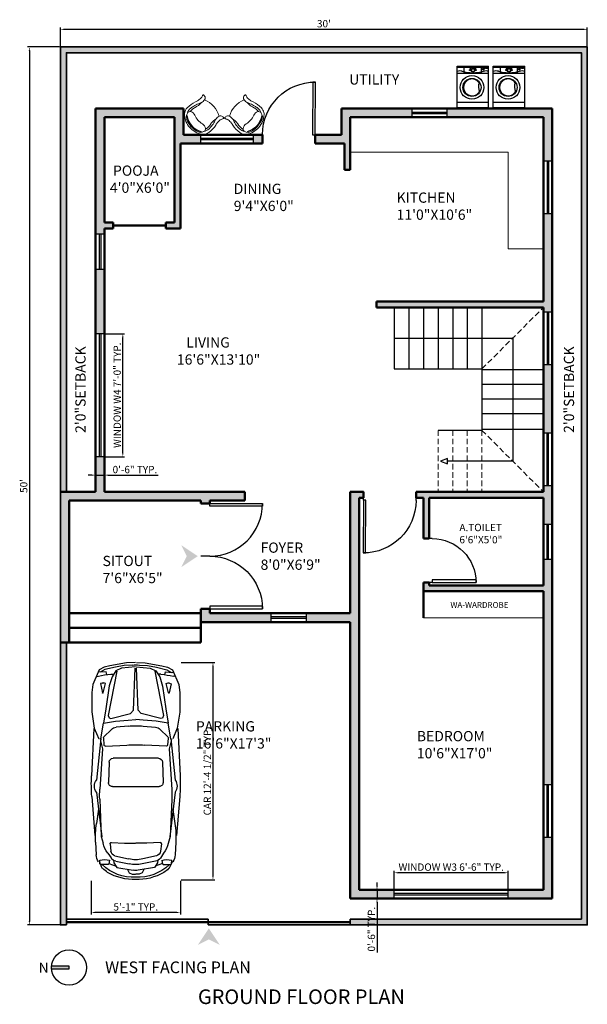
# Model space of a CAD drawing. Units: inches. Extents: x 2638 to 4577, y 1946 to 2619.
# Tile 7 of 8: x 3767 to 4155, y 1946 to 2619. Entities that reach past the tile are written whole.
import ezdxf

# ---------------------------------------------------------------- set-up
doc = ezdxf.new("R2010")
doc.units = ezdxf.units.IN
doc.linetypes.add('DASHED', pattern=[19.05, 12.7, -6.35])
for name, color, linetype, lineweight in [('A-ANNO-DIMS', 2, 'Continuous', 18), ('A-ANNO-SYMB', 1, 'Continuous', 25), ('A-ANNO-TEXT', 7, 'Continuous', 25), ('A-AREA-IDEN', 7, 'Continuous', 25), ('A-DOOR', 4, 'Continuous', 25), ('A-FLOR-FIXT', 8, 'Continuous', 18), ('A-FLOR-OVHD', 8, 'DASHED', 18), ('A-FLOR-STRS', 3, 'Continuous', 25), ('A-FURN', 8, 'Continuous', 18), ('A-GLAZ', 4, 'Continuous', 25), ('A-WALL', 7, 'Continuous', 50), ('A-WALL-PATT', 8, 'Continuous', 13), ('C-PROP', 1, 'Continuous', 35), ('C-PROP-PATT', 252, 'Continuous', 13)]:
    doc.layers.add(name, color=color, linetype=linetype, lineweight=lineweight)
for name, color, linetype in [('IFF-FURN-DETAIL', 250, 'Continuous'), ('L9012X$0', 2, 'Continuous'), ('Сантехника', 7, 'Continuous')]:
    doc.layers.add(name, color=color, linetype=linetype)
doc.styles.get("Standard").update_dxf_attribs({"font": 'arial.ttf'})
doc.dimstyles.new('ISO-25', dxfattribs={"dimtxt": 5, "dimasz": 2.5, "dimexe": 1.25, "dimexo": 0.625, "dimtad": 1, "dimdec": 1, "dimlunit": 3, "dimtxsty": 'Standard', "dimcen": 2.5, "dimclrt": 1, "dimadec": 0, "dimazin": 0, "dimtfac": 1, "dimtdec": 1, "dimtmove": 0, "dimatfit": 3, "dimfxl": 1, "dimarcsym": 0})

# ---------------------------------------------------------------- blocks, each defined once
blk = doc.blocks.new('*D39')
at = {"layer": 'A-ANNO-DIMS', "color": 0, "lineweight": -2, "transparency": 16777216}
for p, q in [((3795, 2600.78), (3795, 2613.44)), ((3797.5, 2612.19), (4152.5, 2612.19)), ((4155, 2600.78), (4155, 2613.44))]:
    blk.add_line(p, q, dxfattribs=at)
at = {"layer": 'A-ANNO-DIMS', "color": 0, "transparency": 16777216}
for points in [[(3797.5, 2612.61), (3797.5, 2611.77), (3795, 2612.19)], [(4152.5, 2612.61), (4152.5, 2611.77), (4155, 2612.19)]]:
    blk.add_solid(points, dxfattribs=at)
at = {"layer": 'Defpoints', "color": 0, "transparency": 16777216}
for p in [(4155, 2612.19), (3795, 2600.16), (4155, 2600.16)]:
    blk.add_point(p, dxfattribs=at)
at = {"layer": 'A-ANNO-DIMS', "color": 0, "transparency": 16777216, "insert": (3975, 2615.37), "char_height": 5, "attachment_point": 5}
blk.add_mtext("30'", dxfattribs=at)
blk = doc.blocks.new('*D40')
at = {"layer": 'A-ANNO-DIMS', "color": 0, "lineweight": -2, "transparency": 16777216}
for p, q in [((3794.38, 2600.16), (3772.46, 2600.16)), ((3773.71, 2597.66), (3773.71, 2002.66)), ((3794.38, 2000.16), (3772.46, 2000.16))]:
    blk.add_line(p, q, dxfattribs=at)
at = {"layer": 'A-ANNO-DIMS', "color": 0, "transparency": 16777216}
for points in [[(3773.29, 2597.66), (3774.12, 2597.66), (3773.71, 2600.16)], [(3773.29, 2002.66), (3774.12, 2002.66), (3773.71, 2000.16)]]:
    blk.add_solid(points, dxfattribs=at)
at = {"layer": 'Defpoints', "color": 0, "transparency": 16777216}
for p in [(3795, 2600.16), (3773.71, 2000.16), (3795, 2000.16)]:
    blk.add_point(p, dxfattribs=at)
at = {"layer": 'A-ANNO-DIMS', "color": 0, "transparency": 16777216, "insert": (3770.53, 2300.16), "char_height": 5, "attachment_point": 5, "rotation": 90}
blk.add_mtext("50'", dxfattribs=at)
blk = doc.blocks.new('*U5')
for p, q in [((0, 0), (0, -6)), ((30, 0), (30, -6))]:
    blk.add_line(p, q)
blk.add_lwpolyline([(0, 0), (0, 30), (1.75, 30), (1.75, 0)], close=True)
blk.add_arc((0, 0), 30, 0, 90)
blk = doc.blocks.new('*U4')
for p, q in [((0, 0), (0, -6)), ((36, 0), (36, -6))]:
    blk.add_line(p, q)
blk.add_lwpolyline([(0, 0), (0, 36), (1.75, 36), (1.75, 0)], close=True)
blk.add_arc((0, 0), 36, 0, 90)
blk = doc.blocks.new('wash')
at = {"layer": 'Сантехника'}
for p, q in [((4817.13, 2840.92), (4788.24, 2840.92)), ((4788.24, 2819.46), (4788.24, 2840.92)), ((4788.93, 2819.46), (4788.93, 2840.92)), ((4793.08, 2819.46), (4793.08, 2840.92)), ((4812.98, 2819.46), (4812.98, 2840.92)), ((4816.44, 2819.46), (4816.44, 2840.92)), ((4817.13, 2819.46), (4817.13, 2840.92)), ((4793.08, 2836.07), (4788.93, 2836.07)), ((4817.13, 2819.46), (4788.24, 2819.46)), ((4793.08, 2824.31), (4788.93, 2824.31)), ((4817.13, 2816.27), (4788.24, 2816.27)), ((4788.24, 2794.82), (4788.24, 2816.27)), ((4788.93, 2794.82), (4788.93, 2816.27)), ((4793.08, 2794.82), (4793.08, 2816.27)), ((4812.98, 2794.82), (4812.98, 2816.27)), ((4816.44, 2794.82), (4816.44, 2816.27)), ((4817.13, 2794.82), (4817.13, 2816.27)), ((4793.08, 2811.43), (4788.93, 2811.43)), ((4793.08, 2799.66), (4788.93, 2799.66)), ((4817.13, 2794.82), (4788.24, 2794.82))]:
    blk.add_line(p, q, dxfattribs=at)
for points in [[(4789.4, 2839.27), (4789.4, 2840.17), (4789.9, 2840.17), (4789.9, 2839.27)], [(4789.4, 2837.95), (4789.4, 2838.85), (4789.9, 2838.85), (4789.9, 2837.95)], [(4789.4, 2836.64), (4789.4, 2837.53), (4789.9, 2837.53), (4789.9, 2836.64)], [(4790.27, 2836.64), (4790.27, 2837.53), (4790.77, 2837.53), (4790.77, 2836.64)], [(4789.4, 2814.62), (4789.4, 2815.52), (4789.9, 2815.52), (4789.9, 2814.62)], [(4789.4, 2813.31), (4789.4, 2814.2), (4789.9, 2814.2), (4789.9, 2813.31)], [(4789.4, 2811.99), (4789.4, 2812.89), (4789.9, 2812.89), (4789.9, 2811.99)], [(4790.27, 2811.99), (4790.27, 2812.89), (4790.77, 2812.89), (4790.77, 2811.99)]]:
    blk.add_lwpolyline(points, close=True, dxfattribs=at)
for centre, radius in [((4802.77, 2829.54), 8.1), ((4802.77, 2829.54), 6.17), ((4789.46, 2831.45), 0.271), ((4789.46, 2828.92), 0.271), ((4790.98, 2830.19), 1.34), ((4790.19, 2831.93), 0.271), ((4790.98, 2830.19), 1.07), ((4790.19, 2828.4), 0.271), ((4790.98, 2832.18), 0.271), ((4790.98, 2828.15), 0.271), ((4802.77, 2804.9), 8.1), ((4789.46, 2806.8), 0.271), ((4790.98, 2805.55), 1.34), ((4790.19, 2807.28), 0.271), ((4790.98, 2805.55), 1.07), ((4790.98, 2807.53), 0.271), ((4802.77, 2804.9), 6.17), ((4789.46, 2804.27), 0.271), ((4790.19, 2803.75), 0.271), ((4790.98, 2803.5), 0.271)]:
    blk.add_circle(centre, radius, dxfattribs=at)
for centre, radius, start, end in [((4796.44, 2838.85), 4.89, 154.89498, 196.60684), ((4762.87, 2829.66), 29.92, 1.02061, 15.09365), ((4802.77, 2829.54), 5.77, 121.80671, 62.15064), ((4802.39, 2840.74), 6.83, 243.19, 300.76734), ((4762.87, 2830.72), 29.92, 344.90635, 358.97939), ((4796.44, 2821.54), 4.89, 163.39316, 205.10502), ((4796.44, 2814.2), 4.89, 154.89498, 196.60684), ((4762.87, 2805.01), 29.92, 1.02061, 15.09365), ((4802.77, 2804.9), 5.77, 121.80671, 62.15064), ((4802.39, 2816.1), 6.83, 243.19, 300.76734), ((4762.87, 2806.08), 29.92, 344.90635, 358.97939), ((4796.44, 2796.89), 4.89, 163.39316, 205.10502)]:
    blk.add_arc(centre, radius, start, end, dxfattribs=at)
blk = doc.blocks.new('ILNG95')
for points in [[(120, 308, -0.32971), (51, 384, -0.036099), (50, 422, -0.497733), (75, 439, -0.070621), (96, 429, 0.101868), (133, 414, 0.091794), (259, 412, 0.024114), (351, 433, -0.090294), (638, 458, -0.132412), (775, 407, -0.068618), (816, 368, -0.184346), (943, 0, 1.803905)], [(120, 308, 0.138132), (244, 313, 0.001085), (325, 339, -0.034227), (462, 375, -0.033255), (567, 387, -0.137428), (727, 350, -4.561553)], [(120, 308, 0.138132), (244, 313, 0.001085), (325, 339, -0.034227), (462, 375, -0.033255), (567, 387, -0.137428), (727, 350, -4.561553)], [(235, 308, 0.064243), (394, 307, 0.04414), (433, 315, -0.118032), (643, 329, -6.296816)], [(235, 308, 0.064243), (394, 307, 0.04414), (433, 315, -0.118032), (643, 329, -6.296816)], [(639, 0, 0.078302), (612, 161, -0.233633), (633, 315, -0.28763), (710, 349, -0.317923), (875, 193, -0.032882), (900, 0, 1.140397)], [(639, 0, 0.078302), (612, 161, -0.233633), (633, 315, -0.28763), (710, 349, -0.317923), (875, 193, -0.032882), (900, 0, 1.140397)], [(120, -308, 0.32971), (51, -384, 0.036099), (50, -422, 0.497733), (75, -439, 0.070621), (96, -429, -0.101868), (133, -414, -0.091794), (259, -412, -0.024114), (351, -433, 0.090294), (638, -458, 0.132412), (775, -407, 0.068618), (816, -368, 0.184346), (943, 0, -1.803905)], [(639, 0, -0.078302), (612, -161, 0.233633), (633, -315, 0.28763), (710, -349, 0.317923), (875, -193, 0.032882), (900, 0, -1.140397)], [(639, 0, -0.078302), (612, -161, 0.233633), (633, -315, 0.28763), (710, -349, 0.317923), (875, -193, 0.032882), (900, 0, -1.140397)], [(120, -308, -0.138132), (244, -313, -0.001085), (325, -339, 0.034227), (462, -375, 0.033255), (567, -387, 0.137428), (727, -350, 4.561553)], [(120, -308, -0.138132), (244, -313, -0.001085), (325, -339, 0.034227), (462, -375, 0.033255), (567, -387, 0.137428), (727, -350, 4.561553)], [(235, -308, -0.064243), (394, -307, -0.04414), (433, -315, 0.118032), (643, -329, 6.296816)], [(235, -308, -0.064243), (394, -307, -0.04414), (433, -315, 0.118032), (643, -329, 6.296816)]]:
    blk.add_lwpolyline(points, format="xyb")
blk.add_arc((759, 1), 709, 154.3281, 205.801)
at = {"layer": 'IFF-FURN-DETAIL'}
blk.add_arc((326, -2), 549, 326.8997, 34.6691, dxfattribs=at)
blk.add_arc((326, -2), 549, 326.8997, 34.6691, dxfattribs=at)
blk = doc.blocks.new('A1099DC')
at = {"color": 0, "linetype": 'ByBlock'}
for p, q in [((1279.298465, 804.448389), (2201.430588, 851.890505)), ((2602.736326, 846.078152), (3356.693814, 785.353187)), ((3488.458929, 772.663345), (3732.658862, 759.86454)), ((92.537504, 388.14361), (139.051458, 595.027331)), ((139.051458, 595.027331), (190.951238, 683.213377)), ((179.200345, 564.515703), (190.951238, 709.631982)), ((272.228253, 749.073842), (265.114727, 718.465169)), ((405.405047, 577.538958), (396.874865, 615.894428)), ((398.733388, 644.315148), (411.280494, 678.748261)), ((589.014326, 626.599587), (405.405047, 577.538958)), ((411.280494, 678.748261), (588.616917, 641.417897)), ((1482.852352, 674.283145), (1175.286956, 622.180789)), ((1300.814287, 466.658131), (1445.712032, 613.104998)), ((1465.665584, 620.56924), (1602.893878, 610.287296)), ((1475.52921, 670.226262), (2282.402739, 758.004075)), ((1494.603245, 682.841284), (1678.210958, 641.166865)), ((1626.354615, 583.507504), (1602.652901, 169.222264)), ((1678.210958, 641.166865), (2462.684993, 690.847736)), ((2519.280414, 756.817792), (3387.476361, 653.818028)), ((2656.476214, 692.831247), (3376.704709, 662.004075)), ((2851.341839, 715.213377), (3126.60716, 755.701993)), ((3376.704709, 662.004075), (3510.708679, 626.736433)), ((3909.27561, 688.812956), (3837.725727, 693.401722)), ((3867.794139, 700.329656), (3900.059395, 686.767505)), ((3921.162781, 527.618662), (3921.162781, 676.138994)), ((3925.383812, 676.122818), (3955.306409, 663.545364)), ((57.774444, 216.608726), (92.537504, 388.14361)), ((236.043912, 551.980927), (179.200345, 564.515703)), ((229.117398, 477.634662), (225.714299, 427.957563)), ((1860.238743, -448.635916), (1859.369151, 433.397797)), ((1933.148906, 509.557888), (2330.980062, 522.200075)), ((2409.60024, 445.938054), (2410.49349, -460.09121)), ((3493.960271, 465.734554), (3507.923021, 209.166865)), ((3522.252709, 492.345257), (3666.066199, 475.644444)), ((3704.596898, 536.993674), (3795.675135, 473.385795)), ((3753.293176, 397.789551), (3815.226005, 132.124765)), ((3839.396146, 426.841284), (3888.358202, 417.538958)), ((3841.786866, 503.451367), (3910.58243, 515.096797)), ((3888.358202, 417.538958), (3983.199613, 359.957848)), ((3901.001848, 514.780764), (3957.150905, 375.772812)), ((49.168662, 58.00681), (57.774444, 216.608726)), ((1235.045743, 136.116317), (1257.419842, 373.755108)), ((3507.923021, 209.166865), (3507.64153, -4.333678)), ((3857.610793, 379.525702), (3912.067615, 118.157673)), ((3983.199613, 359.957848), (4035.448301, 43.94997)), ((4019.086894, 150.376168), (4084.69605, 122.469191)), ((4084.69605, 122.469191), (4109.177079, 60.329656)), ((4109.177079, 60.329656), (4113.094043, -5.158716)), ((49.301278, -76.507426), (58.219773, -235.092064)), ((1235.330373, -152.586046), (1258.173002, -390.180259)), ((1627.520644, -599.204785), (1603.002095, -184.967086)), ((3508.347273, -221.154823), (3507.644805, -7.65525)), ((3754.088875, -409.293325), (3815.497749, -143.506937)), ((3858.370276, -390.823819), (3912.311631, -129.348921)), ((3983.920268, -371.008369), (4035.545755, -54.898082)), ((4019.394229, -161.356334), (4084.948231, -133.320044)), ((4084.948231, -133.320044), (4109.306686, -71.132359)), ((4109.306686, -71.132359), (4113.094514, -5.636391)), ((58.219773, -235.092064), (93.320996, -406.558069)), ((3494.890446, -477.749545), (3508.347273, -221.154823)), ((3889.19258, -428.776374), (3983.920268, -371.008369)), ((93.320996, -406.558069), (140.24279, -613.349673)), ((237.150178, -570.112104), (180.331436, -582.758939)), ((230.077082, -495.779641), (226.576036, -446.109349)), ((1301.750547, -482.997536), (1446.936772, -629.158411)), ((1934.168526, -524.650381), (2332.023837, -536.508105)), ((3523.2353, -504.304409), (3667.01558, -487.320059)), ((3705.667171, -548.593196), (3796.61981, -484.805853)), ((3840.248961, -438.175225), (3889.19258, -428.776374)), ((3842.790735, -514.780444), (3911.609128, -526.290202)), ((3902.027941, -525.993061), (3957.902795, -386.874665)), ((3922.214148, -538.79118), (3922.506998, -687.311224)), ((140.24279, -613.349673), (192.316354, -701.433212)), ((180.331436, -582.758939), (192.368445, -727.851766)), ((273.723073, -767.133288), (266.549207, -736.538701)), ((406.561378, -595.336142), (398.106841, -633.708356)), ((400.0214, -662.125356), (412.636377, -696.533662)), ((590.267037, -644.034637), (406.561378, -595.336142)), ((412.636377, -696.533662), (589.898847, -658.853701)), ((1484.19765, -690.263206), (1176.530118, -638.767405)), ((1466.905004, -636.583294), (1604.112757, -626.030785)), ((1476.866524, -686.22077), (2283.911563, -772.40743)), ((1495.965396, -698.798158), (1679.490579, -656.761786)), ((1679.490579, -656.761786), (2464.061049, -704.895745)), ((2520.786439, -770.754078), (3388.777604, -666.042617)), ((2657.855804, -706.497136), (3378.022114, -674.249887)), ((2852.765183, -728.494989), (3128.109803, -768.440762)), ((3378.022114, -674.249887), (3511.956283, -638.718087)), ((3910.644841, -700.0086), (3839.104145, -704.738438)), ((3869.186159, -711.60707), (3901.424611, -697.981326)), ((3926.727989, -687.286725), (3956.625729, -674.650294)), ((1280.900818, -820.829563), (2203.124693, -866.453338)), ((2604.418191, -859.849707), (3358.254477, -797.638217)), ((3489.994314, -784.688586), (3734.168535, -771.408296))]:
    blk.add_line(p, q, dxfattribs=at)
for points in [[(-0.000783, 0.794772), (5.385043, 172.701749), (63.649891, 493.818028), (92.537504, 603.957563), (144.437284, 705.166865), (428.417214, 824.236633), (585.095796, 846.190121), (961.406447, 846.190121), (1274.27399, 797.818028), (1482.852352, 709.631982)], [(83.345007, -3.206171), (111.32237, 268.957533), (164.563706, 379.583828), (279.999271, 453.709838), (456.549665, 511.628518), (901.254996, 574.918954), (1175.286956, 622.180789), (1137.52997, 385.548359), (1118.345181, 137.317882), (1109.829198, -8.358455)], [(168.178729, 359.003083), (1030.214866, 528.397865), (1077.798844, 510.531569), (1086.170082, 475.285426), (992.832238, 91.960378), (924.218938, 35.478085), (108.447994, 6.034416)], [(0.019119, -19.392451), (5.743899, -191.288474), (64.641806, -512.289243), (93.746535, -622.371603), (145.845778, -723.478374), (430.059935, -841.987962), (586.7815, -863.632471), (963.091723, -863.198028), (1275.863278, -814.209121), (1484.26735, -725.611974)], [(83.356858, -15.227176), (111.870816, -287.335185), (165.330179, -397.856284), (280.911681, -471.754535), (457.575935, -529.324983), (902.4055, -592.045995), (1176.530118, -638.767405), (1138.306616, -402.209884), (1118.632407, -154.017717), (1109.829198, -8.358455)], [(168.904615, -377.268451), (1031.273389, -545.270714), (1078.822046, -527.310627), (1087.123771, -492.048047), (993.030273, -108.907787), (924.305735, -52.560894), (108.478017, -24.418246)]]:
    blk.add_lwpolyline(points, dxfattribs=at)
for centre, radius, start, end in [((2358.037832, -2192.08357), 3048, 85.395244, 92.945173), ((2399.99649, 588.663508), 206.166238, 54.649181, 124.776949), ((3392.740754, -1053.630025), 1828.8, 86.999806, 98.367602), ((1749.553982, 373.478072), 1524, 166.916578, 176.08111), ((446.46332, 626.922805), 50.8, 159.97873, 192.538409), ((587.047263, 633.961317), 7.62, 284.960009, 78.112462), ((1463.767788, 595.240237), 25.4, 85.715073, 135.304647), ((1600.996082, 584.958293), 25.4, 356.725615, 85.715073), ((2578.271641, -1134.295865), 1828.8, 87.549126, 93.623712), ((3355.555414, 37.211519), 609.6, 55.070043, 75.255062), ((3718.678317, 475.802507), 284.405862, 57.329946, 87.182375), ((4191.049821, 605.937201), 363.988953, 166.096081, 196.353514), ((3908.462781, 676.138994), 12.7, 0, 86.330429), ((3320.85101, 50.338397), 847.430844, 356.245089, 44.519453), ((3896.252417, 523.051998), 152.4, 46.38363, 67.20138), ((3700.933354, 318.064082), 435.542335, 30.457681, 46.38363), ((1409.148822, 359.469565), 152.4, 135.304647, 174.62136), ((1935.569151, 433.396333), 76.2, 91.82012, 179.9989), ((2333.400307, 446.03852), 76.2, 359.924458, 91.82012), ((3519.322741, 467.114813), 25.4, 83.37601, 183.115039), ((3654.346327, 374.722669), 101.6, 13.122645, 83.37601), ((3708.414764, 348.440256), 152.4, 11.769371, 55.070043), ((3908.462781, 527.618662), 12.7, 279.607718, 0), ((3204.184594, 25.950693), 1011.814461, 358.069446, 30.457681), ((1266.577845, -8.050136), 1219.2, 176.894161, 183.218814), ((2752.335538, -6.739118), 1524, 174.62136, 185.491615), ((4645.676894, -4.872483), 3048, 176.725615, 183.38736), ((3221.54491, -6.276527), 609.6, 346.99033, 13.122645), ((3315.283499, -6.18411), 609.6, 348.343604, 11.769371), ((3734.73098, -5.770579), 304.8, 350.724636, 9.388339), ((3320.962449, -62.69553), 847.430844, 315.593523, 3.867886), ((3204.248172, -38.537915), 1011.814461, 329.655294, 2.043529), ((1750.305335, -388.625277), 1524, 184.031865, 193.196397), ((1409.873518, -375.595566), 152.4, 185.491615, 224.808328), ((1936.438592, -448.484202), 76.2, 180.114076, 268.292856), ((2334.293902, -460.341926), 76.2, 268.292856, 0.188517), ((3520.255588, -479.079792), 25.4, 176.997936, 276.736965), ((3355.640902, -49.500248), 609.6, 284.857913, 305.042932), ((3655.096735, -386.42159), 101.6, 276.736965, 346.99033), ((3709.113243, -360.032616), 152.4, 305.042932, 348.343604), ((4192.255091, -616.577407), 363.988953, 163.759461, 194.016894), ((3909.514173, -538.816222), 12.7, 0.112975, 80.505257), ((3701.571953, -329.671253), 435.542335, 313.729345, 329.655294), ((447.716945, -644.638934), 50.8, 167.574566, 200.134245), ((588.314493, -651.400231), 7.62, 282.000513, 75.152966), ((1464.957267, -611.258083), 25.4, 224.808328, 274.397903), ((1602.165021, -600.705574), 25.4, 274.397903, 3.38736), ((2576.048678, 1120.472221), 1828.8, 266.489263, 272.563849), ((3719.627907, -487.374382), 284.405862, 272.930601, 302.78303), ((3909.807023, -687.336265), 12.7, 273.782546, 0.112975), ((3897.294828, -534.273643), 152.4, 292.911596, 313.729345), ((2353.729565, 2177.823616), 3048, 267.167802, 274.717731), ((2401.171182, -602.835323), 206.166238, 235.336026, 305.463794), ((3390.675263, 1041.412497), 1828.8, 261.745373, 273.113169)]:
    blk.add_arc(centre, radius, start, end, dxfattribs=at)
blk = doc.blocks.new('VI')
at = {"layer": 'L9012X$0'}
blk.add_blockref('A1099DC', (0, 0), dxfattribs=at)
blk = doc.blocks.new('WIN-36')
for p, q in [((2761.41, 2540.16), (2761.41, 2534.16)), ((2761.41, 2537.66), (2797.41, 2537.66)), ((2761.41, 2536.66), (2797.41, 2536.66)), ((2797.41, 2540.16), (2797.41, 2534.16))]:
    blk.add_line(p, q)
blk = doc.blocks.new('WIN-24')
for p, q in [((2905.41, 2558.16), (2905.41, 2552.16)), ((2929.41, 2558.16), (2929.41, 2552.16)), ((2905.41, 2555.66), (2929.41, 2555.66)), ((2905.41, 2554.66), (2929.41, 2554.66))]:
    blk.add_line(p, q)
blk = doc.blocks.new('WIN-84')
for p, q in [((2695.41, 2404.16), (2689.41, 2404.16)), ((2691.91, 2404.16), (2691.91, 2320.16)), ((2692.91, 2404.16), (2692.91, 2320.16)), ((2695.41, 2320.16), (2689.41, 2320.16))]:
    blk.add_line(p, q)
blk = doc.blocks.new('WIN-78')
for p, q in [((3314.99, 2024.16), (3314.99, 2018.16)), ((3314.99, 2021.66), (3392.99, 2021.66)), ((3314.99, 2020.66), (3392.99, 2020.66)), ((3392.99, 2024.16), (3392.99, 2018.16))]:
    blk.add_line(p, q)
blk = doc.blocks.new('*D51')
at = {"layer": 'A-ANNO-DIMS', "color": 0, "lineweight": -2, "transparency": 16777216}
for p, q in [((4023, 2024.78), (4023, 2037.11)), ((4098.5, 2035.86), (4025.5, 2035.86)), ((4101, 2024.78), (4101, 2037.11))]:
    blk.add_line(p, q, dxfattribs=at)
at = {"layer": 'A-ANNO-DIMS', "color": 0, "transparency": 16777216}
for points in [[(4025.5, 2036.27), (4025.5, 2035.44), (4023, 2035.86)], [(4098.5, 2036.27), (4098.5, 2035.44), (4101, 2035.86)]]:
    blk.add_solid(points, dxfattribs=at)
at = {"layer": 'Defpoints', "color": 0, "transparency": 16777216}
for p in [(4023, 2035.86), (4023, 2024.16), (4101, 2024.16)]:
    blk.add_point(p, dxfattribs=at)
at = {"layer": 'A-ANNO-DIMS', "color": 1, "transparency": 16777216, "insert": (4062, 2039.07), "char_height": 5, "attachment_point": 5}
blk.add_mtext('WINDOW W3 6\'-6" TYP.', dxfattribs=at)
blk = doc.blocks.new('*D52')
at = {"layer": 'A-ANNO-DIMS', "color": 0, "lineweight": -2, "transparency": 16777216}
for p, q in [((4011.3, 2026.66), (4011.3, 2029.16)), ((4022.38, 2024.16), (4010.05, 2024.16)), ((4011.3, 2024.16), (4011.3, 2018.16)), ((4022.38, 2018.16), (4010.05, 2018.16)), ((4011.3, 2015.66), (4011.3, 1981.43))]:
    blk.add_line(p, q, dxfattribs=at)
at = {"layer": 'A-ANNO-DIMS', "color": 0, "transparency": 16777216}
for points in [[(4010.89, 2026.66), (4011.72, 2026.66), (4011.3, 2024.16)], [(4010.89, 2015.66), (4011.72, 2015.66), (4011.3, 2018.16)]]:
    blk.add_solid(points, dxfattribs=at)
at = {"layer": 'Defpoints', "color": 0, "transparency": 16777216}
for p in [(4023, 2024.16), (4011.3, 2018.16), (4023, 2018.16)]:
    blk.add_point(p, dxfattribs=at)
at = {"layer": 'A-ANNO-DIMS', "color": 1, "transparency": 16777216, "insert": (4008.12, 1997.29), "char_height": 5, "attachment_point": 5, "rotation": 90}
blk.add_mtext('0\'-6" TYP.', dxfattribs=at)
blk = doc.blocks.new('*D53')
at = {"layer": 'A-ANNO-DIMS', "color": 0, "lineweight": -2, "transparency": 16777216}
for p, q in [((3825.63, 2404.16), (3838.85, 2404.16)), ((3837.6, 2322.66), (3837.6, 2401.66)), ((3825.63, 2320.16), (3838.85, 2320.16))]:
    blk.add_line(p, q, dxfattribs=at)
at = {"layer": 'A-ANNO-DIMS', "color": 0, "transparency": 16777216}
for points in [[(3837.19, 2401.66), (3838.02, 2401.66), (3837.6, 2404.16)], [(3837.19, 2322.66), (3838.02, 2322.66), (3837.6, 2320.16)]]:
    blk.add_solid(points, dxfattribs=at)
at = {"layer": 'Defpoints', "color": 0, "transparency": 16777216}
for p in [(3825, 2404.16), (3837.6, 2404.16), (3825, 2320.16)]:
    blk.add_point(p, dxfattribs=at)
at = {"layer": 'A-ANNO-DIMS', "color": 1, "transparency": 16777216, "insert": (3834.39, 2362.16), "char_height": 5, "attachment_point": 5, "rotation": 90}
blk.add_mtext('WINDOW W4 7\'-0" TYP.', dxfattribs=at)
blk = doc.blocks.new('*D54')
at = {"layer": 'A-ANNO-DIMS', "color": 0, "lineweight": -2, "transparency": 16777216}
for p, q in [((3819, 2319.53), (3819, 2306.31)), ((3825, 2319.53), (3825, 2306.31)), ((3816.5, 2307.56), (3814, 2307.56)), ((3819, 2307.56), (3825, 2307.56)), ((3827.5, 2307.56), (3861.73, 2307.56))]:
    blk.add_line(p, q, dxfattribs=at)
at = {"layer": 'A-ANNO-DIMS', "color": 0, "transparency": 16777216}
for points in [[(3816.5, 2307.97), (3816.5, 2307.14), (3819, 2307.56)], [(3827.5, 2307.97), (3827.5, 2307.14), (3825, 2307.56)]]:
    blk.add_solid(points, dxfattribs=at)
at = {"layer": 'Defpoints', "color": 0, "transparency": 16777216}
for p in [(3819, 2320.16), (3825, 2320.16), (3825, 2307.56)]:
    blk.add_point(p, dxfattribs=at)
at = {"layer": 'A-ANNO-DIMS', "color": 1, "transparency": 16777216, "insert": (3845.87, 2310.73), "char_height": 5, "attachment_point": 5}
blk.add_mtext('0\'-6" TYP.', dxfattribs=at)
blk = doc.blocks.new('*D81')
at = {"layer": 'A-ANNO-DIMS', "color": 0, "lineweight": -2, "transparency": 16777216}
for p, q in [((3877.54, 2179.54), (3900.45, 2179.54)), ((3899.2, 2177.04), (3899.2, 2033.46)), ((3877.54, 2030.96), (3900.45, 2030.96))]:
    blk.add_line(p, q, dxfattribs=at)
at = {"layer": 'A-ANNO-DIMS', "color": 0, "transparency": 16777216}
for points in [[(3898.79, 2177.04), (3899.62, 2177.04), (3899.2, 2179.54)], [(3898.79, 2033.46), (3899.62, 2033.46), (3899.2, 2030.96)]]:
    blk.add_solid(points, dxfattribs=at)
at = {"layer": 'Defpoints', "color": 0, "transparency": 16777216}
for p in [(3876.92, 2179.54), (3876.92, 2030.96), (3899.2, 2030.96)]:
    blk.add_point(p, dxfattribs=at)
at = {"layer": 'A-ANNO-DIMS', "color": 1, "transparency": 16777216, "insert": (3895.99, 2105.25), "char_height": 5, "attachment_point": 5, "rotation": 90}
blk.add_mtext('CAR 12\'-4 1/2" TYP.', dxfattribs=at)
blk = doc.blocks.new('*D82')
at = {"layer": 'A-ANNO-DIMS', "color": 0, "lineweight": -2, "transparency": 16777216}
for p, q in [((3815.97, 2030.33), (3815.97, 2007.42)), ((3876.92, 2030.33), (3876.92, 2007.42)), ((3874.42, 2008.67), (3818.47, 2008.67))]:
    blk.add_line(p, q, dxfattribs=at)
at = {"layer": 'A-ANNO-DIMS', "color": 0, "transparency": 16777216}
for points in [[(3818.47, 2009.09), (3818.47, 2008.25), (3815.97, 2008.67)], [(3874.42, 2009.09), (3874.42, 2008.25), (3876.92, 2008.67)]]:
    blk.add_solid(points, dxfattribs=at)
at = {"layer": 'Defpoints', "color": 0, "transparency": 16777216}
for p in [(3815.97, 2030.96), (3876.92, 2030.96), (3815.97, 2008.67)]:
    blk.add_point(p, dxfattribs=at)
at = {"layer": 'A-ANNO-DIMS', "color": 1, "transparency": 16777216, "insert": (3846.45, 2011.85), "char_height": 5, "attachment_point": 5}
blk.add_mtext('5\'-1" TYP.', dxfattribs=at)

msp = doc.modelspace()

# ---------------------------------------------------------------- hatches: boundary and pattern name
at = {"layer": 'A-ANNO-SYMB', "transparency": 33554687}
h = msp.add_hatch(color=256, dxfattribs=at)
h.dxf.hatch_style = 1
h.paths.add_polyline_path([(3881.24, 2252.16), (3877.47, 2244.61), (3888.79, 2252.16), (3877.47, 2259.71)])
h = msp.add_hatch(color=256, dxfattribs=at)
h.dxf.hatch_style = 1
h.paths.add_polyline_path([(3896.39, 1990.28), (3903.94, 1986.51), (3896.39, 1997.83), (3888.84, 1986.51)])
h = msp.add_hatch(color=256, dxfattribs=at)
h.dxf.hatch_style = 1
h.paths.add_polyline_path([(3800.82, 1972.11), (3800.82, 1970.11), (3788.86, 1970.11, -0.020861), (3788.82, 1971.11, -0.020861), (3788.86, 1972.11)])
at = {"layer": 'A-WALL-PATT', "transparency": 33554687}
h = msp.add_hatch(color=256, dxfattribs=at)
h.dxf.hatch_style = 1
h.paths.add_polyline_path([(3879, 2558.16), (3819, 2558.16), (3819, 2472.16), (3825, 2472.16), (3825, 2476.16), (3831, 2476.16), (3831, 2480.16), (3825, 2480.16), (3825, 2552.16), (3873, 2552.16), (3873, 2480.16), (3867, 2480.16), (3867, 2476.16), (3877, 2476.16), (3877, 2534.16), (3891, 2534.16), (3891, 2540.16), (3879, 2540.16)])
h.paths.add_polyline_path([(3933, 2540.16), (3927, 2540.16), (3927, 2534.16), (3933, 2534.16)])
h.paths.add_polyline_path([(4035, 2558.16), (3987, 2558.16), (3987, 2540.16), (3969.04, 2540.16), (3969.04, 2540.16), (3969, 2534.26), (3969, 2534.16), (3989, 2534.16), (3989, 2516.16), (3993, 2516.16), (3993, 2552.16), (4035, 2552.16)])
h.paths.add_polyline_path([(4131, 2558.16), (4059, 2558.16), (4059, 2552.16), (4125, 2552.16), (4125, 2522.16), (4131, 2522.16)])
h.paths.add_polyline_path([(4131, 2486.16), (4125, 2486.16), (4125, 2426.16), (4011, 2426.16), (4011, 2422.16), (4125, 2422.16), (4125, 2418.91), (4131, 2418.91)])
h.paths.add_polyline_path([(4131, 2382.91), (4125, 2382.91), (4125, 2336.41), (4131, 2336.41)])
h.paths.add_polyline_path([(4131, 2300.41), (4125, 2300.41), (4125, 2296.16), (4038, 2296.16), (4038, 2292.16), (4043, 2292.16), (4043, 2264.16), (4047, 2264.16), (4047, 2292.16), (4125, 2292.16), (4125, 2274.16), (4131, 2274.16)])
h.paths.add_polyline_path([(4131, 2250.16), (4125, 2250.16), (4125, 2232.16), (4047, 2232.16), (4047, 2234.16), (4043, 2234.16), (4043, 2228.16), (4125, 2228.16), (4125, 2096.16), (4131, 2096.16)])
h.paths.add_polyline_path([(4131, 2060.16), (4125, 2060.16), (4125, 2024.16), (4101, 2024.16), (4101, 2018.16), (4131, 2018.16)])
h.paths.add_polyline_path([(3999, 2292.16), (4002, 2292.16), (4002, 2296.16), (3993, 2296.16), (3993, 2213.16), (3963, 2213.16), (3963, 2207.16), (3993, 2207.16), (3993, 2018.16), (4023, 2018.16), (4023, 2024.16), (3999, 2024.16)])
h.paths.add_polyline_path([(3939, 2213.16), (3897, 2213.16), (3897, 2216.16), (3891, 2216.16), (3891, 2207.16), (3939, 2207.16)])
h.paths.add_polyline_path([(3801, 2290.16), (3891, 2290.16), (3891, 2288.16), (3897, 2288.16), (3897, 2290.16), (3921, 2290.16), (3921, 2296.16), (3825, 2296.16), (3825, 2320.16), (3819, 2320.16), (3819, 2296.16), (3795, 2296.16), (3795, 2193.16), (3801, 2193.16)])
h.paths.add_polyline_path([(3825, 2448.16), (3819, 2448.16), (3819, 2404.16), (3825, 2404.16)])
at = {"layer": 'C-PROP-PATT', "transparency": 33554687}
h = msp.add_hatch(color=256, dxfattribs=at)
h.dxf.hatch_style = 1
h.paths.add_polyline_path([(4155, 2600.16), (3795, 2600.16), (3795, 2296.16), (3799, 2296.16), (3799, 2596.16), (4151, 2596.16), (4151, 2004.16), (3993, 2004.16), (3993, 2000.16), (4155, 2000.16)])
h.paths.add_polyline_path([(3799, 2193.16), (3795, 2193.16), (3795, 2000.16), (3799, 2000.16)], flags=17)

# ---------------------------------------------------------------- linework, layer by layer
at = {"layer": 'A-ANNO-SYMB'}
for p, q in [((3800.82, 1972.11), (3788.86, 1972.11)), ((3800.82, 1970.11), (3800.82, 1972.11)), ((3788.82, 1970.11), (3800.82, 1970.11))]:
    msp.add_line(p, q, dxfattribs=at)
msp.add_circle((3800.82, 1971.11), 12, dxfattribs=at)
at = {"layer": 'A-FLOR-FIXT'}
for p, q in [((3993, 2528.16), (4101, 2528.16)), ((4101, 2528.16), (4101, 2462.16)), ((4101, 2462.16), (4125, 2462.16))]:
    msp.add_line(p, q, dxfattribs=at)
at = {"layer": 'A-FLOR-OVHD', "ltscale": 0.3}
for p, q in [((4083, 2380.16), (4125, 2422.16)), ((4053, 2338.16), (4053, 2296.16)), ((4063, 2338.16), (4063, 2296.16)), ((4073, 2338.16), (4073, 2296.16)), ((4083, 2338.16), (4083, 2296.16)), ((4083, 2338.16), (4125, 2296.16))]:
    msp.add_line(p, q, dxfattribs=at)
at = {"layer": 'A-FLOR-STRS'}
for p, q in [((4023, 2422.16), (4023, 2380.16)), ((4033, 2422.16), (4033, 2380.16)), ((4043, 2422.16), (4043, 2380.16)), ((4053, 2422.16), (4053, 2380.16)), ((4063, 2422.16), (4063, 2380.16)), ((4073, 2422.16), (4073, 2380.16)), ((4083, 2422.16), (4083, 2338.16)), ((4023, 2380.16), (4083, 2380.16)), ((4083, 2379.66), (4125, 2379.66)), ((4083, 2369.66), (4125, 2369.66)), ((4083, 2359.66), (4125, 2359.66)), ((4083, 2349.66), (4125, 2349.66)), ((4083, 2338.16), (4053, 2338.16)), ((4125, 2338.66), (4083, 2338.66))]:
    msp.add_line(p, q, dxfattribs=at)
msp.add_lwpolyline([(4023, 2401.16), (4104, 2401.16), (4104, 2317.16), (4059.4, 2317.16)], dxfattribs=at)
msp.add_lwpolyline([(4054.63, 2317.16), (4059.4, 2315.29), (4059.4, 2319.03)], close=True, dxfattribs=at)
at = {"layer": 'A-FURN'}
for p, q in [((3831, 2478.66), (3849, 2478.66)), ((3849, 2478.66), (3849, 2477.66)), ((3849, 2477.66), (3867, 2477.66)), ((4125, 2210.16), (4043, 2210.16))]:
    msp.add_line(p, q, dxfattribs=at)
at = {"layer": 'A-WALL'}
for p, q in [((3819, 2558.16), (3879, 2558.16)), ((3819, 2296.16), (3819, 2558.16)), ((3879, 2540.16), (3879, 2558.16)), ((3987, 2558.16), (4131, 2558.16)), ((3987, 2558.16), (3987, 2540.16)), ((4131, 2558.16), (4131, 2018.16)), ((3825, 2552.16), (3873, 2552.16)), ((3825, 2480.16), (3825, 2552.16)), ((3873, 2480.16), (3873, 2552.16)), ((3993, 2552.16), (4125, 2552.16)), ((3993, 2552.16), (3993, 2516.16)), ((4125, 2552.16), (4125, 2426.16)), ((3879, 2540.16), (3933, 2540.16)), ((3933, 2540.16), (3933, 2534.16)), ((3969, 2540.16), (3987, 2540.16)), ((3969, 2540.16), (3969, 2534.16)), ((3877, 2534.16), (3933, 2534.16)), ((3877, 2476.16), (3877, 2534.16)), ((3969, 2534.16), (3989, 2534.16)), ((3989, 2534.16), (3989, 2516.16)), ((3989, 2516.16), (3993, 2516.16)), ((3825, 2480.16), (3831, 2480.16)), ((3825, 2476.16), (3831, 2476.16)), ((3825, 2296.16), (3825, 2476.16)), ((3831, 2480.16), (3831, 2476.16)), ((3831, 2478.16), (3867, 2478.16)), ((3867, 2480.16), (3873, 2480.16)), ((3867, 2480.16), (3867, 2476.16)), ((3867, 2476.16), (3877, 2476.16)), ((4011, 2426.16), (4125, 2426.16)), ((4011, 2426.16), (4011, 2422.16)), ((4011, 2422.16), (4125, 2422.16)), ((4125, 2422.16), (4125, 2296.16)), ((3819, 2296.16), (3795, 2296.16)), ((3921, 2296.16), (3825, 2296.16)), ((3921, 2296.16), (3921, 2290.16)), ((3993, 2296.16), (3993, 2213.16)), ((4002, 2296.16), (3993, 2296.16)), ((4002, 2296.16), (4002, 2292.16)), ((4125, 2296.16), (4038, 2296.16)), ((4038, 2296.16), (4038, 2292.16)), ((3891, 2290.16), (3801, 2290.16)), ((3801, 2193.16), (3801, 2290.16)), ((3891, 2290.16), (3891, 2288.16)), ((3897, 2288.16), (3891, 2288.16)), ((3897, 2290.16), (3897, 2288.16)), ((3921, 2290.16), (3897, 2290.16)), ((3999, 2292.16), (3999, 2024.16)), ((4002, 2292.16), (3999, 2292.16)), ((4043, 2292.16), (4038, 2292.16)), ((4043, 2292.16), (4043, 2264.16)), ((4125, 2292.16), (4047, 2292.16)), ((4047, 2292.16), (4047, 2264.16)), ((4125, 2292.16), (4125, 2232.16)), ((4047, 2264.16), (4043, 2264.16)), ((4043, 2234.16), (4043, 2210.16)), ((4047, 2234.16), (4043, 2234.16)), ((4047, 2234.16), (4047, 2232.16)), ((4125, 2228.16), (4043, 2228.16)), ((4125, 2232.16), (4047, 2232.16)), ((4125, 2228.16), (4125, 2024.16)), ((3891, 2216.16), (3891, 2193.16)), ((3897, 2216.16), (3891, 2216.16)), ((3897, 2216.16), (3897, 2213.16)), ((3891, 2213.16), (3801, 2213.16)), ((3993, 2207.16), (3891, 2207.16)), ((3993, 2213.16), (3897, 2213.16)), ((3993, 2207.16), (3993, 2018.16)), ((3891, 2203.16), (3801, 2203.16)), ((3891, 2193.16), (3795, 2193.16)), ((4125, 2024.16), (3999, 2024.16)), ((4131, 2018.16), (3993, 2018.16)), ((3993, 2002.16), (3799, 2002.16))]:
    msp.add_line(p, q, dxfattribs=at)
at = {"layer": 'C-PROP'}
for p, q in [((3799, 2004.16), (3896, 2004.16)), ((3896, 2002.16), (3896, 2004.16)), ((3896, 2002.16), (3896, 2000.16)), ((3993, 2000.16), (3896, 2000.16)), ((3993, 2004.16), (3993, 2000.16))]:
    msp.add_line(p, q, dxfattribs=at)
for points in [[(3799, 2000.16), (3795, 2000.16), (3795, 2600.16), (4155, 2600.16), (4155, 2000.16), (3993, 2000.16)], [(3799, 2296.16), (3799, 2596.16), (4151, 2596.16), (4151, 2004.16), (3993, 2004.16)], [(3799, 2000.16), (3799, 2193.16)]]:
    msp.add_lwpolyline(points, dxfattribs=at)

# ---------------------------------------------------------------- block references
at = {"layer": 'A-DOOR', "xscale": -1}
for name, p, rotation in [('*U4', (3969.04, 2540.16), 359.6786649249896), ('*U4', (4001.97, 2290.36), 179.6786649249896), ('*U5', (4049, 2234.16), 270), ('*U4', (3897, 2216.16), 270)]:
    msp.add_blockref(name, p, dxfattribs=dict(at, rotation=rotation))
at = {"layer": 'A-DOOR', "rotation": 270}
msp.add_blockref('*U4', (3897, 2288.16), dxfattribs=at)
at = {"layer": 'A-FLOR-FIXT', "rotation": 270}
msp.add_blockref('wash', (1271.29, 7375.29), dxfattribs=at)
at = {"layer": 'A-FURN'}
for name, p, xscale, yscale, zscale, rotation in [('ILNG95', (3900.61, 2560.38), 0.0243705291132055, 0.0243705291132055, 0.0243705291132055, 221.4118781376283), ('ILNG95', (3913.25, 2560.38), -0.0243705291132055, 0.0243705291132055, 0.0243705291132055, 138.5881218623715), ('VI', (3846.19, 2179.54), -0.0351896714874634, 0.0351896714874634, 0.0351896714874634, 90)]:
    msp.add_blockref(name, p, dxfattribs=dict(at, xscale=xscale, yscale=yscale, zscale=zscale, rotation=rotation))
at = {"layer": 'A-GLAZ'}
for name in ['WIN-24', 'WIN-84']:
    msp.add_blockref(name, (1129.59, 0), dxfattribs=at)
for name, p, rotation in [('WIN-36', (6688.41, 5074.31), 180), ('WIN-36', (1590.85, 5283.57), 270.0000000000028), ('WIN-24', (1266.85, 5377.57), 270.0000000000102), ('WIN-36', (1590.85, 5180.32), 270.0000000000031), ('WIN-36', (6665.16, -461), 90.00000000000541), ('WIN-24', (6683.16, -655.25), 90.00000000001023), ('WIN-24', (6868.41, 4765.31), 180), ('WIN-36', (6665.16, -701.25), 90.00000000000561), ('WIN-78', (7415.99, 4042.31), 180)]:
    msp.add_blockref(name, p, dxfattribs=dict(at, rotation=rotation))

# ---------------------------------------------------------------- texts
at = {"layer": 'A-ANNO-SYMB'}
msp.add_text('N', height=6.9, dxfattribs=at).set_placement((3780.08, 1967.57))
at = {"layer": 'A-ANNO-TEXT', "attachment_point": 1}
for s, width, insert, char_height in [('{\\fTimes New Roman|b0|i0|c0|p18;UTILITY}', 61.0557, (3992.3, 2581.44), 7), ('WA-WARDROBE', 29.5334, (4061.46, 2220.86), 4), ('{\\fTimes New Roman|b0|i0|c0|p18;WEST FACING PLAN}', 196.2607, (3825.51, 1975.23), 8), ('{\\fTimes New Roman|b0|i0|c0|p18;GROUND FLOOR PLAN}', 196.2607, (3888.92, 1956.14), 10)]:
    msp.add_mtext_dynamic_manual_height_columns(s, width=width, gutter_width=12.5, heights=[0], dxfattribs=dict(at, insert=insert, char_height=char_height))
at = {"layer": 'A-ANNO-TEXT', "char_height": 7, "attachment_point": 1, "rotation": 90}
for insert in [(3805.16, 2336.4), (4138.97, 2336.4)]:
    msp.add_mtext_dynamic_manual_height_columns('{\\fTimes New Roman|b0|i0|c0|p18;2\'0"SETBACK}', width=61.0557, gutter_width=12.5, heights=[0], dxfattribs=dict(at, insert=insert))
at = {"layer": 'A-AREA-IDEN', "attachment_point": 1}
for s, insert, char_height in [('{\\fTimes New Roman|b0|i0|c0|p18; POOJA\\P4\'0"X6\'0"}', (3828.75, 2519.14), 7), ('{\\fTimes New Roman|b0|i0|c0|p18;DINING\\P9\'4"X6\'0"}', (3913.39, 2506.69), 7), ('{\\fTimes New Roman|b0|i0|c0|p18;KITCHEN\\P11\'0"X10\'6"}', (4024.7, 2500.7), 7), ('{\\fTimes New Roman|b0|i0|c0|p18;   LIVING\\P16\'6"X13\'10"}', (3874.56, 2401.74), 7), ('{\\fTimes New Roman|b0|i0|c0|p18;A.TOILET\\P6\'6"X5\'0"}', (4067.62, 2274.28), 5), ('{\\fTimes New Roman|b0|i0|c0|p18;FOYER\\P8\'0"X6\'9"}', (3931.74, 2261.53), 7), ('{\\fTimes New Roman|b0|i0|c0|p18;SITOUT\\P7\'6"X6\'5"}', (3823.75, 2252.43), 7), ('{\\fTimes New Roman|b0|i0|c0|p18;PARKING\\P16\'6"X17\'3"}', (3887.52, 2139.41), 7), ('{\\fTimes New Roman|b0|i0|c0|p18;BEDROOM\\P10\'6"X17\'0"}', (4038.53, 2132.7), 7)]:
    msp.add_mtext_dynamic_manual_height_columns(s, width=61.0557, gutter_width=12.5, heights=[0], dxfattribs=dict(at, insert=insert, char_height=char_height))

# ---------------------------------------------------------------- dimensions: what is measured, and where the dimension line sits
at = {"layer": 'A-ANNO-DIMS'}
dim = msp.add_linear_dim(base=(4155, 2612.19), p1=(3795, 2600.16), p2=(4155, 2600.16), dimstyle='ISO-25', override={"dimclrd": 0, "dimclre": 0, "dimclrt": 0}, dxfattribs=at)
dim.commit()
dim.dimension.update_dxf_attribs({"geometry": '*D39', "text_midpoint": (3975, 2615.37)})
dim = msp.add_linear_dim(base=(3773.71, 2000.16), p1=(3795, 2600.16), p2=(3795, 2000.16), angle=90, dimstyle='ISO-25', override={"dimclrd": 0, "dimclre": 0, "dimclrt": 0}, dxfattribs=at)
dim.commit()
dim.dimension.update_dxf_attribs({"geometry": '*D40', "text_midpoint": (3770.53, 2300.16)})
for base, p1, p2, angle, text, picture, middle in [((3837.6, 2404.16), (3825, 2320.16), (3825, 2404.16), 90, 'WINDOW W4 <> TYP.', '*D53', (3834.39, 2362.16)), ((3899.2, 2030.96), (3876.92, 2179.54), (3876.92, 2030.96), 270, 'CAR <> TYP.', '*D81', (3895.99, 2105.25)), ((4023, 2035.86), (4101, 2024.16), (4023, 2024.16), 180, 'WINDOW W3 <> TYP.', '*D51', (4062, 2039.07)), ((3815.9748, 2008.6697), (3876.9178, 2030.9567), (3815.9748, 2030.9567), 180, '<> TYP.', '*D82', (3846.4463, 2011.8475)), ((4011.3, 2018.16), (4023, 2024.16), (4023, 2018.16), 270, '<> TYP.', '*D52', (4008.12, 1997.29))]:
    dim = msp.add_linear_dim(base=base, p1=p1, p2=p2, angle=angle, text=text, dimstyle='ISO-25', override={"dimdec": 1, "dimrnd": 0, "dimzin": 1, "dimlunit": 4, "dimfrac": 2}, dxfattribs=at)
    dim.commit()
    dim.dimension.update_dxf_attribs({"geometry": picture, "text_midpoint": middle})
dim = msp.add_linear_dim(base=(3825, 2307.56), p1=(3819, 2320.16), p2=(3825, 2320.16), text='<> TYP.', dimstyle='ISO-25', override={"dimdec": 1, "dimrnd": 0, "dimzin": 1, "dimlunit": 4, "dimfrac": 2}, dxfattribs=at)
dim.commit()
dim.dimension.update_dxf_attribs({"geometry": '*D54', "text_midpoint": (3845.87, 2310.73)})

doc.saveas('drawing.dxf')
